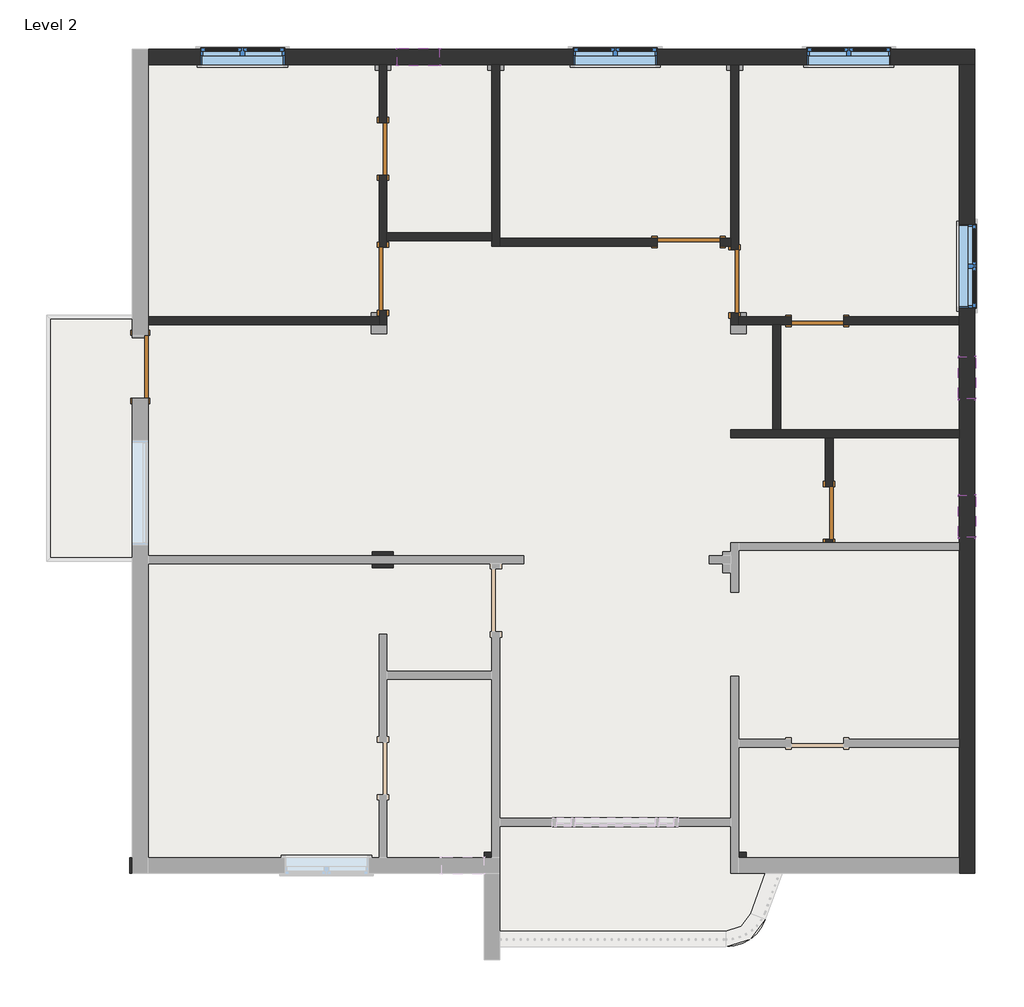
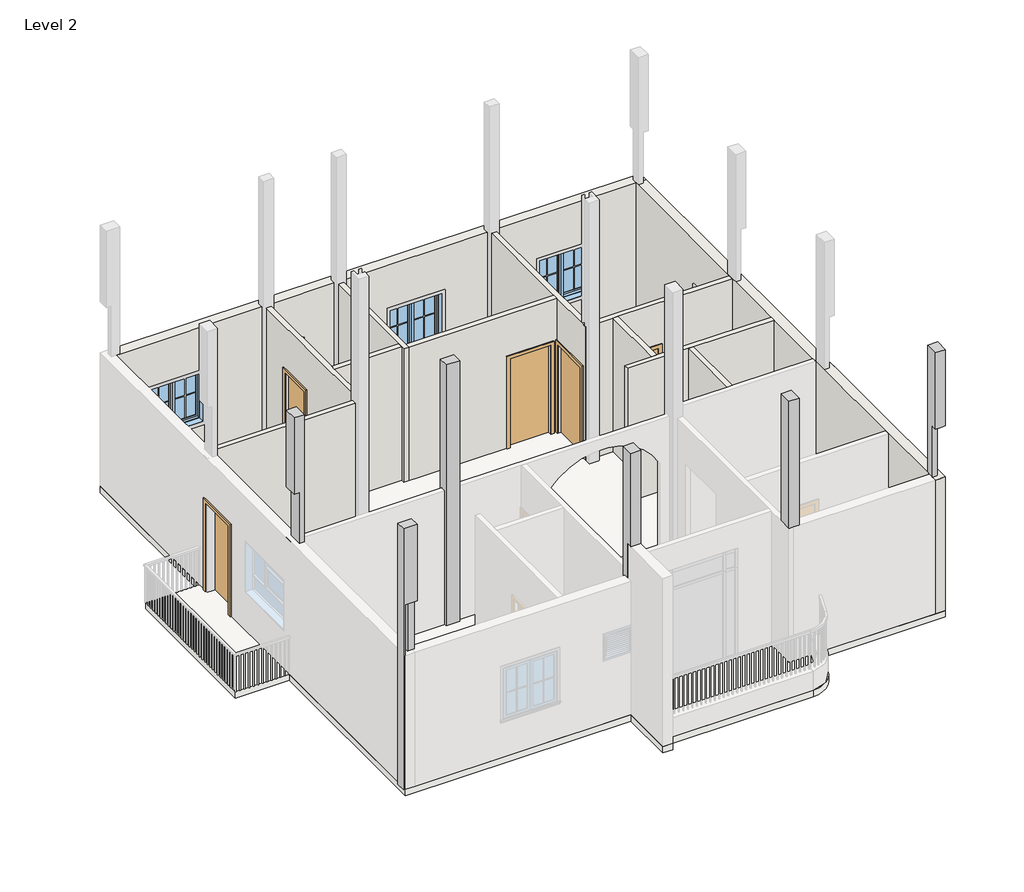
# One storey, part 2 of 4: 12 walls, 7 doors, 7 windows, 6 columns, 1 slab.
"""IFC4 building model written with IfcOpenShell, lengths in millimetres."""

from ifc_helpers import new_model, si_unit, point, frame, frame_2d, origin, place, context, project, spatial, polyline, circle_curve, trimmed, segment, composite_curve, outline, extrude, faceted_brep, transform, mapped, element, save
from components import door_78caadf7, door_214872d5, door_305aa2a5, door_e5f9f3c4, door_a90ba1ad, window_af3140d2, window_f2d8fef0

model = new_model("IFC4")

# Units and contexts
model_context = context("Model", 3, world=origin())
ifc_project = project(units=[si_unit("LENGTHUNIT", "METRE", prefix="MILLI")], contexts=[model_context])

# Site, building, storey
site = spatial("IfcSite", under=ifc_project)
building = spatial("IfcBuilding", under=site)
storey = spatial("IfcBuildingStorey", under=building, Name="Level 2", Elevation=3200.4)

# Columns
placement = place(None, origin())
element("IfcColumn", 1, ObjectType="Rectangular Column : 9\" x 12\"", at=placement, inside=storey, context=model_context, shape_type="Brep", body=[
    faceted_brep([(-14895.9678125, 6235.466018, 3200.4), (-14667.3678125, 6235.466018, 3200.4), (-14667.3678125, 6178.316018, 3200.4), (-14667.3678125, 6064.016018, 3200.4), (-14667.3678125, 5930.666018, 3200.4), (-14895.9678125, 5930.666018, 3200.4), (-14895.9678125, 6235.466018, 6400.8), (-14781.6678125, 6235.466018, 6400.8), (-14781.6678125, 6235.466018, 7620.0), (-14895.9678125, 6235.466018, 7620.0), (-14895.9678125, 6235.466018, 9448.8), (-14667.3678125, 6235.466018, 9448.8), (-14667.3678125, 5930.666018, 9448.8), (-14895.9678125, 5930.666018, 9448.8), (-14895.9678125, 5930.666018, 7620.0), (-14781.6678125, 5930.666018, 7620.0), (-14781.6678125, 5930.666018, 6400.8), (-14895.9678125, 5930.666018, 6400.8)], [[[0, 1, 2, 3, 4, 5]], [[1, 0, 6, 7, 8, 9, 10, 11]], [[4, 3, 2, 1, 11, 12]], [[5, 4, 12, 13, 14, 15, 16, 17]], [[13, 10, 9, 14]], [[11, 10, 13, 12]], [[7, 16, 15, 8]], [[16, 7, 6, 17]], [[8, 15, 14, 9]], [[0, 5, 17, 6]]]),
])
element("IfcColumn", 2, ObjectType="Rectangular Column : 9\" x 12\"", at=placement, inside=storey, context=model_context, shape_type="SweptSolid", body=[
    extrude(outline(polyline([(6006.866018, 3200.4), (6006.866018, 9448.8), (6235.466018, 9448.8), (6235.466018, 3200.4), (6178.316018, 3200.4), (6178.316018, 6400.8), (6064.016018, 6400.8), (6064.016018, 3200.4), (6006.866018, 3200.4)])), frame((-11409.8178125, 0.0, 0.0), z_axis=(1.0, 0.0, 0.0), x_axis=(0.0, 1.0, 0.0)), (0.0, 0.0, 1.0), 304.8),
])
element("IfcColumn", 3, ObjectType="Rectangular Column : 9\" x 12\"", at=placement, inside=storey, context=model_context, shape_type="Brep", body=[
    faceted_brep([(-14934.0678125, 1568.216018, 3200.4), (-14934.0678125, 1796.816018, 3200.4), (-14895.9678125, 1796.816018, 3200.4), (-14895.9678125, 1568.216018, 3200.4), (-14629.2678125, 1796.816018, 9448.8), (-14629.2678125, 1568.216018, 9448.8), (-14629.2678125, 1568.216018, 7620.0), (-14629.2678125, 1682.516018, 7620.0), (-14629.2678125, 1682.516018, 6400.8), (-14629.2678125, 1796.816018, 6400.8), (-14934.0678125, 1568.216018, 9448.8), (-14895.9678125, 1568.216018, 6400.8), (-14895.9678125, 1568.216018, 7620.0), (-14934.0678125, 1796.816018, 9448.8), (-14667.3678125, 1796.816018, 6400.8), (-14781.6678125, 1796.816018, 6400.8), (-14781.6678125, 1796.816018, 7620.0), (-14895.9678125, 1796.816018, 7620.0), (-14895.9678125, 1796.816018, 6400.8), (-14895.9678125, 1682.516018, 6400.8), (-14667.3678125, 1682.516018, 6400.8), (-14781.6678125, 1682.516018, 6400.8), (-14781.6678125, 1682.516018, 7620.0), (-14895.9678125, 1682.516018, 7620.0)], [[[0, 1, 2, 3]], [[4, 5, 6, 7, 8, 9]], [[5, 10, 0, 3, 11, 12, 6]], [[1, 0, 10, 13]], [[1, 13, 4, 9, 14, 15, 16, 17, 18, 2]], [[5, 4, 13, 10]], [[3, 2, 18, 19, 11]], [[14, 20, 21, 15]], [[14, 9, 8, 20]], [[8, 7, 22, 21, 20]], [[7, 6, 12, 23, 22]], [[23, 12, 11, 19]], [[17, 23, 19, 18]], [[22, 16, 15, 21]], [[23, 17, 16, 22]]]),
])
element("IfcColumn", 4, ObjectType="Rectangular Column : 9\" x 12\"", at=placement, inside=storey, context=model_context, shape_type="Brep", body=[
    faceted_brep([(-9561.9678125, 1568.216018, 3200.4), (-9790.5678125, 1568.216018, 3200.4), (-9790.5678125, 1873.016018, 3200.4), (-9676.2678125, 1873.016018, 3200.4), (-9676.2678125, 1796.816018, 3200.4), (-9561.9678125, 1796.816018, 3200.4), (-9790.5678125, 1873.016018, 9448.8), (-9561.9678125, 1873.016018, 9448.8), (-9561.9678125, 1873.016018, 6400.8), (-9676.2678125, 1873.016018, 6400.8), (-9561.9678125, 1568.216018, 9448.8), (-9561.9678125, 1568.216018, 7218.0977729), (-9561.9678125, 1682.516018, 7218.0977729), (-9561.9678125, 1682.516018, 6400.8), (-9561.9678125, 1568.216018, 6400.8), (-9561.9678125, 1796.816018, 6400.8), (-9790.5678125, 1568.216018, 9448.8), (-9790.5678125, 1568.216018, 7620.0), (-9790.5678125, 1568.216018, 7218.0977729), (-9790.5678125, 1568.216018, 6400.8), (-9790.5678125, 1682.516018, 6400.8), (-9790.5678125, 1682.516018, 7218.0977729), (-9676.2678125, 1796.816018, 6400.8)], [[[0, 1, 2, 3, 4, 5]], [[6, 7, 8, 9, 3, 2]], [[7, 10, 11, 12, 13, 14, 0, 5, 15, 8]], [[10, 16, 17, 18, 11]], [[2, 1, 19, 20, 21, 18, 17, 16, 6]], [[7, 6, 16, 10]], [[22, 4, 3, 9]], [[15, 22, 9, 8]], [[4, 22, 15, 5]], [[21, 12, 11, 18]], [[13, 20, 19, 14]], [[12, 21, 20, 13]], [[1, 0, 14, 19]]]),
])
element("IfcColumn", 5, ObjectType="Rectangular Column : 9\" x 12\"", at=placement, inside=storey, context=model_context, shape_type="Brep", body=[
    faceted_brep([(-6094.8678125, 1873.016018, 3200.4), (-5980.5678125, 1873.016018, 3200.4), (-5980.5678125, 1796.816018, 3200.4), (-6094.8678125, 1796.816018, 3200.4), (-6209.1678125, 1873.016018, 9448.8), (-5980.5678125, 1873.016018, 9448.8), (-6094.8678125, 1873.016018, 6400.8), (-6209.1678125, 1873.016018, 6400.8), (-5980.5678125, 1568.216018, 9448.8), (-5980.5678125, 1568.216018, 6400.8), (-5980.5678125, 1796.816018, 6400.8), (-6209.1678125, 1568.216018, 9448.8), (-6209.1678125, 1568.216018, 6400.8), (-6094.8678125, 1568.216018, 6400.8), (-6094.8678125, 1796.816018, 6400.8)], [[[0, 1, 2, 3]], [[4, 5, 1, 0, 6, 7]], [[1, 5, 8, 9, 10, 2]], [[8, 11, 12, 13, 9]], [[11, 4, 7, 12]], [[5, 4, 11, 8]], [[6, 0, 3, 14]], [[7, 6, 14, 13, 12]], [[10, 14, 3, 2]], [[14, 10, 9, 13]]]),
])
element("IfcColumn", 6, ObjectType="Rectangular Column : 9\" x 12\"", at=placement, inside=storey, context=model_context, shape_type="Brep", body=[
    faceted_brep([(-2894.4678125, 1873.016018, 3200.4), (-2665.8678125, 1873.016018, 3200.4), (-2665.8678125, 1568.216018, 3200.4), (-2894.4678125, 1568.216018, 3200.4), (-2894.4678125, 1796.816018, 3200.4), (-2894.4678125, 1873.016018, 9448.8), (-2665.8678125, 1873.016018, 9448.8), (-2665.8678125, 1873.016018, 7620.0), (-2780.1678125, 1873.016018, 7620.0), (-2780.1678125, 1873.016018, 6400.8), (-2665.8678125, 1873.016018, 6400.8), (-2665.8678125, 1568.216018, 9448.8), (-2665.8678125, 1568.216018, 7620.0), (-2894.4678125, 1568.216018, 9448.8), (-2894.4678125, 1568.216018, 7620.0), (-2780.1678125, 1568.216018, 7620.0), (-2894.4678125, 1568.216018, 6400.8), (-2894.4678125, 1682.516018, 6400.8), (-2894.4678125, 1682.516018, 7620.0), (-2780.1678125, 1682.516018, 7620.0), (-2780.1678125, 1682.516018, 6400.8), (-2780.1678125, 1568.216018, 6400.8), (-2665.8678125, 1568.216018, 6400.8)], [[[0, 1, 2, 3, 4]], [[1, 0, 5, 6, 7, 8, 9, 10]], [[6, 11, 12, 7]], [[11, 13, 14, 15, 12]], [[0, 4, 3, 16, 17, 18, 14, 13, 5]], [[6, 5, 13, 11]], [[9, 8, 19, 20]], [[10, 9, 20, 21, 22]], [[8, 7, 12, 15, 19]], [[2, 1, 10, 22]], [[17, 20, 19, 18]], [[20, 17, 16, 21]], [[18, 19, 15, 14]], [[3, 2, 22, 21, 16]]]),
])

# Doors
door_shape = door_78caadf7(model_context)
element("IfcDoor", 7, ObjectType="Single-Flush : 2'6\"x 7'", at=placement, inside=storey, context=model_context, shape_type="MappedRepresentation", body=[
    mapped(door_shape, transform((-11257.4178125, 12083.816018, 3200.4), x_axis=(0.0, 1.0, 0.0), y_axis=(-1.0, 0.0, 0.0), z_axis=(0.0, 0.0, 1.0))),
])
door_2_shape = door_214872d5(model_context)
element("IfcDoor", 8, ObjectType="Single-Flush : 2'6\"x 7'", at=placement, inside=storey, context=model_context, shape_type="MappedRepresentation", body=[
    mapped(door_2_shape, transform((-4951.8678125, 9588.266018, 3200.4), x_axis=(-1.0, 0.0, 0.0), y_axis=(0.0, -1.0, 0.0), z_axis=(0.0, 0.0, 1.0))),
])
element("IfcDoor", 9, ObjectType="Single-Flush : 2'6\"x 7'", at=placement, inside=storey, context=model_context, shape_type="MappedRepresentation", body=[
    mapped(door_2_shape, transform((-4780.4178125, 6800.616018, 3200.4), x_axis=(0.0, -1.0, 0.0), y_axis=(1.0, 0.0, 0.0), z_axis=(0.0, 0.0, 1.0))),
])
door_3_shape = door_305aa2a5(model_context)
element("IfcDoor", 10, ObjectType="Single-Flush : 36\" x 84\"", at=placement, inside=storey, context=model_context, shape_type="MappedRepresentation", body=[
    mapped(door_3_shape, transform((-11257.4178125, 10197.866018, 3200.4), x_axis=(0.0, -1.0, 0.0), y_axis=(1.0, 0.0, 0.0), z_axis=(0.0, 0.0, 1.0))),
])
door_4_shape = door_e5f9f3c4(model_context)
element("IfcDoor", 11, ObjectType="Single-Flush : 36\" x 84\"", at=placement, inside=storey, context=model_context, shape_type="MappedRepresentation", body=[
    mapped(door_4_shape, transform((-6818.7678125, 10731.266018, 3200.4), x_axis=(1.0, 0.0, 0.0), y_axis=(0.0, 1.0, 0.0), z_axis=(0.0, 0.0, 1.0))),
])
element("IfcDoor", 12, ObjectType="Single-Flush : 36\" x 84\"", at=placement, inside=storey, context=model_context, shape_type="MappedRepresentation", body=[
    mapped(door_4_shape, transform((-6152.0178125, 10159.766018, 3200.4), x_axis=(0.0, -1.0, 0.0), y_axis=(1.0, 0.0, 0.0), z_axis=(0.0, 0.0, 1.0))),
])
door_5_shape = door_a90ba1ad(model_context)
element("IfcDoor", 13, ObjectType="Single-Flush : 36\" x 84\"", at=placement, inside=storey, context=model_context, shape_type="MappedRepresentation", body=[
    mapped(door_5_shape, transform((-14781.6678125, 8921.516018, 3200.4), x_axis=(0.0, 1.0, 0.0), y_axis=(-1.0, 0.0, 0.0), z_axis=(0.0, 0.0, 1.0))),
])

# Slab
element("IfcSlab", 14, ObjectType="6\" floor", at=placement, inside=storey, context=model_context, shape_type="SweptSolid", body=[
    extrude(outline(composite_curve([segment(polyline([(-2665.8678125, 13531.616018), (-2665.8678125, 1568.216018), (-5463.3133278, 1568.216018), (-5705.6066674, 902.5205386)]), True, "CONTINUOUS"), segment(trimmed(circle_curve(frame_2d((-6278.443289, 1111.016018)), 609.6), [point((-5705.6066674, 902.5205386))], [point((-6278.443289, 501.416018))], False, "CARTESIAN"), True, "CONTINUOUS"), segment(polyline([(-6278.443289, 501.416018), (-9561.9678125, 501.416018), (-9561.9678125, 310.916018), (-9790.5678125, 310.916018), (-9790.5678125, 1568.216018), (-14895.9678125, 1568.216018), (-14895.9678125, 6121.166018), (-16115.1678125, 6121.166018), (-16115.1678125, 9645.416018), (-14895.9678125, 9645.416018), (-14895.9678125, 13531.616018), (-2665.8678125, 13531.616018)]), True, "CONTINUOUS")], self_intersect=False)), frame((0.0, 0.0, 3048.0), z_axis=(0.0, 0.0, 1.0), x_axis=(1.0, 0.0, 0.0)), (0.0, 0.0, 1.0), 152.4),
])

# Walls
element("IfcWall", 15, ObjectType="4.5\" wall", at=placement, inside=storey, context=model_context, shape_type="Brep", body=[
    faceted_brep([(-11314.5678125, 9740.666018, 5334.0), (-11314.5678125, 9740.666018, 3200.4), (-11314.5678125, 9702.566018, 3200.4), (-11314.5678125, 9645.416018, 3200.4), (-11314.5678125, 9531.116018, 3200.4), (-11314.5678125, 9531.116018, 6400.8), (-11314.5678125, 9645.416018, 6400.8), (-11314.5678125, 9702.566018, 6400.8), (-11314.5678125, 13226.816018, 6400.8), (-11314.5678125, 13303.016018, 6400.8), (-11314.5678125, 13303.016018, 3200.4), (-11314.5678125, 13226.816018, 3200.4), (-11314.5678125, 12464.816018, 3200.4), (-11314.5678125, 12464.816018, 5334.0), (-11314.5678125, 11702.816018, 5334.0), (-11314.5678125, 11702.816018, 3200.4), (-11314.5678125, 10655.066018, 3200.4), (-11314.5678125, 10655.066018, 5334.0), (-11200.2678125, 9531.116018, 3200.4), (-11200.2678125, 9740.666018, 3200.4), (-11200.2678125, 9740.666018, 5334.0), (-11200.2678125, 10655.066018, 5334.0), (-11200.2678125, 10655.066018, 3200.4), (-11200.2678125, 10750.316018, 3200.4), (-11200.2678125, 10864.616018, 3200.4), (-11200.2678125, 11702.816018, 3200.4), (-11200.2678125, 11702.816018, 5334.0), (-11200.2678125, 12464.816018, 5334.0), (-11200.2678125, 12464.816018, 3200.4), (-11200.2678125, 13226.816018, 3200.4), (-11200.2678125, 13303.016018, 3200.4), (-11200.2678125, 13303.016018, 6400.8), (-11200.2678125, 13226.816018, 6400.8), (-11200.2678125, 10864.616018, 6400.8), (-11200.2678125, 10750.316018, 6400.8), (-11200.2678125, 9702.566018, 6400.8), (-11200.2678125, 9683.516018, 6400.8), (-11200.2678125, 9569.216018, 6400.8), (-11200.2678125, 9531.116018, 6400.8)], [[[0, 1, 2, 3, 4, 5, 6, 7, 8, 9, 10, 11, 12, 13, 14, 15, 16, 17]], [[18, 19, 20, 21, 22, 23, 24, 25, 26, 27, 28, 29, 30, 31, 32, 33, 34, 35, 36, 37, 38]], [[16, 15, 25, 24, 23, 22]], [[4, 3, 2, 1, 19, 18]], [[30, 29, 28, 12, 11, 10]], [[9, 8, 7, 6, 5, 38, 37, 36, 35, 34, 33, 32, 31]], [[10, 9, 31, 30]], [[5, 4, 18, 38]], [[13, 12, 28, 27]], [[14, 13, 27, 26]], [[15, 14, 26, 25]], [[20, 19, 1, 0]], [[21, 20, 0, 17]], [[22, 21, 17, 16]]]),
])
element("IfcWall", 16, ObjectType="4.5\" wall", at=placement, inside=storey, context=model_context, shape_type="Brep", body=[
    faceted_brep([(-14667.3678125, 9531.116018, 3200.4), (-11428.8678125, 9531.116018, 3200.4), (-11314.5678125, 9531.116018, 3200.4), (-11314.5678125, 9531.116018, 6400.8), (-11428.8678125, 9531.116018, 6400.8), (-14667.3678125, 9531.116018, 6400.8), (-14667.3678125, 9645.416018, 3200.4), (-14667.3678125, 9645.416018, 6400.8), (-11428.8678125, 9645.416018, 6400.8), (-11371.7178125, 9645.416018, 6400.8), (-11314.5678125, 9645.416018, 6400.8), (-11314.5678125, 9645.416018, 3200.4), (-11428.8678125, 9645.416018, 3200.4)], [[[0, 1, 2, 3, 4, 5]], [[6, 7, 8, 9, 10, 11, 12]], [[2, 1, 0, 6, 12, 11]], [[5, 4, 3, 10, 9, 8, 7]], [[0, 5, 7, 6]], [[3, 2, 11, 10]]]),
])
element("IfcWall", 17, ObjectType="4.5\" wall", at=placement, inside=storey, context=model_context, shape_type="Brep", body=[
    faceted_brep([(-9676.2678125, 13303.016018, 3200.4), (-9676.2678125, 13226.816018, 3200.4), (-9676.2678125, 10864.616018, 3200.4), (-9676.2678125, 10750.316018, 3200.4), (-9676.2678125, 10674.116018, 3200.4), (-9676.2678125, 10674.116018, 6400.8), (-9676.2678125, 10750.316018, 6400.8), (-9676.2678125, 10864.616018, 6400.8), (-9676.2678125, 13226.816018, 6400.8), (-9676.2678125, 13303.016018, 6400.8), (-9561.9678125, 13303.016018, 3200.4), (-9561.9678125, 13303.016018, 6400.8), (-9561.9678125, 13226.816018, 6400.8), (-9561.9678125, 10788.416018, 6400.8), (-9561.9678125, 10674.116018, 6400.8), (-9561.9678125, 10674.116018, 3200.4), (-9561.9678125, 10788.416018, 3200.4), (-9561.9678125, 13226.816018, 3200.4)], [[[0, 1, 2, 3, 4, 5, 6, 7, 8, 9]], [[10, 11, 12, 13, 14, 15, 16, 17]], [[4, 3, 2, 1, 0, 10, 17, 16, 15]], [[9, 8, 7, 6, 5, 14, 13, 12, 11]], [[0, 9, 11, 10]], [[5, 4, 15, 14]]]),
])
element("IfcWall", 18, ObjectType="4.5\" wall", at=placement, inside=storey, context=model_context, shape_type="SweptSolid", body=[
    extrude(outline(polyline([(-9676.2678125, 10750.316018), (-11200.2678125, 10750.316018), (-11200.2678125, 10864.616018), (-9676.2678125, 10864.616018), (-9676.2678125, 10750.316018)])), frame((0.0, 0.0, 3200.4), z_axis=(0.0, 0.0, 1.0), x_axis=(1.0, 0.0, 0.0)), (0.0, 0.0, 1.0), 3200.4),
])
element("IfcWall", 19, ObjectType="4.5\" wall", at=placement, inside=storey, context=model_context, shape_type="Brep", body=[
    faceted_brep([(-6209.1678125, 9702.566018, 5334.0), (-6209.1678125, 9702.566018, 3200.4), (-6209.1678125, 9531.116018, 3200.4), (-6209.1678125, 9531.116018, 6400.8), (-6209.1678125, 9569.216018, 6400.8), (-6209.1678125, 9683.516018, 6400.8), (-6209.1678125, 9702.566018, 6400.8), (-6209.1678125, 10674.116018, 6400.8), (-6209.1678125, 10788.416018, 6400.8), (-6209.1678125, 13226.816018, 6400.8), (-6209.1678125, 13303.016018, 6400.8), (-6209.1678125, 13303.016018, 3200.4), (-6209.1678125, 13226.816018, 3200.4), (-6209.1678125, 10788.416018, 3200.4), (-6209.1678125, 10674.116018, 3200.4), (-6209.1678125, 10616.966018, 3200.4), (-6209.1678125, 10616.966018, 5334.0), (-6094.8678125, 9531.116018, 3200.4), (-6094.8678125, 9645.416018, 3200.4), (-6094.8678125, 9702.566018, 3200.4), (-6094.8678125, 9702.566018, 5334.0), (-6094.8678125, 10616.966018, 5334.0), (-6094.8678125, 10616.966018, 3200.4), (-6094.8678125, 13226.816018, 3200.4), (-6094.8678125, 13303.016018, 3200.4), (-6094.8678125, 13303.016018, 6400.8), (-6094.8678125, 13226.816018, 6400.8), (-6094.8678125, 9702.566018, 6400.8), (-6094.8678125, 9683.516018, 6400.8), (-6094.8678125, 9645.416018, 6400.8), (-6094.8678125, 9531.116018, 6400.8)], [[[0, 1, 2, 3, 4, 5, 6, 7, 8, 9, 10, 11, 12, 13, 14, 15, 16]], [[17, 18, 19, 20, 21, 22, 23, 24, 25, 26, 27, 28, 29, 30]], [[2, 1, 19, 18, 17]], [[15, 14, 13, 12, 11, 24, 23, 22]], [[10, 9, 8, 7, 6, 5, 4, 3, 30, 29, 28, 27, 26, 25]], [[11, 10, 25, 24]], [[3, 2, 17, 30]], [[20, 19, 1, 0]], [[21, 20, 0, 16]], [[22, 21, 16, 15]]]),
])
element("IfcWall", 20, ObjectType="4.5\" wall", at=placement, inside=storey, context=model_context, shape_type="SweptSolid", body=[
    extrude(outline(polyline([(5334.0, -6361.5678125), (3200.4, -6361.5678125), (3200.4, -6209.1678125), (6400.8, -6209.1678125), (6400.8, -9561.9678125), (3200.4, -9561.9678125), (3200.4, -7275.9678125), (5334.0, -7275.9678125), (5334.0, -6361.5678125)])), frame((0.0, 10674.116018, 0.0), z_axis=(0.0, 1.0, 0.0), x_axis=(0.0, 0.0, 1.0)), (0.0, 0.0, 1.0), 114.3),
])
element("IfcWall", 21, ObjectType="4.5\" wall", at=placement, inside=storey, context=model_context, shape_type="Brep", body=[
    faceted_brep([(-6094.8678125, 9531.116018, 3200.4), (-5980.5678125, 9531.116018, 3200.4), (-5599.5678125, 9531.116018, 3200.4), (-5485.2678125, 9531.116018, 3200.4), (-5332.8678125, 9531.116018, 3200.4), (-5332.8678125, 9531.116018, 5334.0), (-4570.8678125, 9531.116018, 5334.0), (-4570.8678125, 9531.116018, 3200.4), (-2894.4678125, 9531.116018, 3200.4), (-2894.4678125, 9531.116018, 6400.8), (-5485.2678125, 9531.116018, 6400.8), (-5599.5678125, 9531.116018, 6400.8), (-5980.5678125, 9531.116018, 6400.8), (-6094.8678125, 9531.116018, 6400.8), (-5332.8678125, 9645.416018, 5334.0), (-5332.8678125, 9645.416018, 3200.4), (-5980.5678125, 9645.416018, 3200.4), (-6094.8678125, 9645.416018, 3200.4), (-6094.8678125, 9645.416018, 6400.8), (-6037.7178125, 9645.416018, 6400.8), (-5980.5678125, 9645.416018, 6400.8), (-2894.4678125, 9645.416018, 6400.8), (-2894.4678125, 9645.416018, 3200.4), (-4570.8678125, 9645.416018, 3200.4), (-4570.8678125, 9645.416018, 5334.0)], [[[0, 1, 2, 3, 4, 5, 6, 7, 8, 9, 10, 11, 12, 13]], [[14, 15, 16, 17, 18, 19, 20, 21, 22, 23, 24]], [[23, 22, 8, 7]], [[17, 16, 15, 4, 3, 2, 1, 0]], [[13, 12, 11, 10, 9, 21, 20, 19, 18]], [[0, 13, 18, 17]], [[9, 8, 22, 21]], [[5, 4, 15, 14]], [[6, 5, 14, 24]], [[7, 6, 24, 23]]]),
])
element("IfcWall", 22, ObjectType="4.5\" wall", at=placement, inside=storey, context=model_context, shape_type="Brep", body=[
    faceted_brep([(-2894.4678125, 8007.116018, 3200.4), (-5485.2678125, 8007.116018, 3200.4), (-5599.5678125, 8007.116018, 3200.4), (-6209.1678125, 8007.116018, 3200.4), (-6209.1678125, 8007.116018, 6400.8), (-5599.5678125, 8007.116018, 6400.8), (-5485.2678125, 8007.116018, 6400.8), (-2894.4678125, 8007.116018, 6400.8), (-2894.4678125, 7892.816018, 3200.4), (-2894.4678125, 7892.816018, 6400.8), (-4723.2678125, 7892.816018, 6400.8), (-4837.5678125, 7892.816018, 6400.8), (-6209.1678125, 7892.816018, 6400.8), (-6209.1678125, 7892.816018, 3200.4), (-4837.5678125, 7892.816018, 3200.4), (-4723.2678125, 7892.816018, 3200.4)], [[[0, 1, 2, 3, 4, 5, 6, 7]], [[8, 9, 10, 11, 12, 13, 14, 15]], [[3, 2, 1, 0, 8, 15, 14, 13]], [[4, 3, 13, 12]], [[7, 6, 5, 4, 12, 11, 10, 9]], [[0, 7, 9, 8]]]),
])
element("IfcWall", 23, ObjectType="4.5\" wall", at=placement, inside=storey, context=model_context, shape_type="SweptSolid", body=[
    extrude(outline(polyline([(-5599.5678125, 8007.116018), (-5599.5678125, 9531.116018), (-5485.2678125, 9531.116018), (-5485.2678125, 8007.116018), (-5599.5678125, 8007.116018)])), frame((0.0, 0.0, 3200.4), z_axis=(0.0, 0.0, 1.0), x_axis=(1.0, 0.0, 0.0)), (0.0, 0.0, 1.0), 3200.4),
])
element("IfcWall", 24, ObjectType="4.5\" wall", at=placement, inside=storey, context=model_context, shape_type="SweptSolid", body=[
    extrude(outline(polyline([(6419.616018, 5334.0), (6419.616018, 3200.4), (6368.816018, 3200.4), (6368.816018, 6400.8), (7892.816018, 6400.8), (7892.816018, 3200.4), (7181.616018, 3200.4), (7181.616018, 5334.0), (6419.616018, 5334.0)])), frame((-4837.5678125, 0.0, 0.0), z_axis=(1.0, 0.0, 0.0), x_axis=(0.0, 1.0, 0.0)), (0.0, 0.0, 1.0), 114.3),
])
element("IfcWall", 25, ObjectType="9\" wall", at=placement, inside=storey, context=model_context, shape_type="Brep", body=[
    faceted_brep([(-14667.3678125, 13303.016018, 3200.4), (-14591.1678125, 13303.016018, 3200.4), (-11371.7178125, 13303.016018, 3200.4), (-11314.5678125, 13303.016018, 3200.4), (-11200.2678125, 13303.016018, 3200.4), (-11143.1178125, 13303.016018, 3200.4), (-9733.4178125, 13303.016018, 3200.4), (-9676.2678125, 13303.016018, 3200.4), (-9561.9678125, 13303.016018, 3200.4), (-9504.8178125, 13303.016018, 3200.4), (-6266.3178125, 13303.016018, 3200.4), (-6209.1678125, 13303.016018, 3200.4), (-6094.8678125, 13303.016018, 3200.4), (-6037.7178125, 13303.016018, 3200.4), (-2894.4678125, 13303.016018, 3200.4), (-2665.8678125, 13303.016018, 3200.4), (-2665.8678125, 13303.016018, 6400.8), (-2780.1678125, 13303.016018, 6400.8), (-2894.4678125, 13303.016018, 6400.8), (-6037.7178125, 13303.016018, 6400.8), (-6094.8678125, 13303.016018, 6400.8), (-6209.1678125, 13303.016018, 6400.8), (-6266.3178125, 13303.016018, 6400.8), (-9504.8178125, 13303.016018, 6400.8), (-9561.9678125, 13303.016018, 6400.8), (-9676.2678125, 13303.016018, 6400.8), (-9733.4178125, 13303.016018, 6400.8), (-11143.1178125, 13303.016018, 6400.8), (-11200.2678125, 13303.016018, 6400.8), (-11314.5678125, 13303.016018, 6400.8), (-11371.7178125, 13303.016018, 6400.8), (-14591.1678125, 13303.016018, 6400.8), (-14667.3678125, 13303.016018, 6400.8), (-10438.2678125, 13303.016018, 5334.0), (-10438.2678125, 13303.016018, 4724.4), (-11047.8678125, 13303.016018, 4724.4), (-11047.8678125, 13303.016018, 5334.0), (-12686.1678125, 13303.016018, 5334.0), (-12686.1678125, 13303.016018, 4114.8), (-13905.3678125, 13303.016018, 4114.8), (-13905.3678125, 13303.016018, 5334.0), (-7275.9678125, 13303.016018, 5334.0), (-7275.9678125, 13303.016018, 4114.8), (-8495.1678125, 13303.016018, 4114.8), (-8495.1678125, 13303.016018, 5334.0), (-3885.0678125, 13303.016018, 5334.0), (-3885.0678125, 13303.016018, 4114.8), (-5104.2678125, 13303.016018, 4114.8), (-5104.2678125, 13303.016018, 5334.0), (-14667.3678125, 13531.616018, 3200.4), (-14667.3678125, 13531.616018, 6400.8), (-2665.8678125, 13531.616018, 6400.8), (-2665.8678125, 13531.616018, 3200.4), (-14591.1678125, 13531.616018, 3200.4), (-10438.2678125, 13531.616018, 5334.0), (-11047.8678125, 13531.616018, 5334.0), (-11047.8678125, 13531.616018, 4724.4), (-10438.2678125, 13531.616018, 4724.4), (-12686.1678125, 13531.616018, 5334.0), (-13905.3678125, 13531.616018, 5334.0), (-13905.3678125, 13531.616018, 4114.8), (-12686.1678125, 13531.616018, 4114.8), (-7275.9678125, 13531.616018, 5334.0), (-8495.1678125, 13531.616018, 5334.0), (-8495.1678125, 13531.616018, 4114.8), (-7275.9678125, 13531.616018, 4114.8), (-3885.0678125, 13531.616018, 5334.0), (-5104.2678125, 13531.616018, 5334.0), (-5104.2678125, 13531.616018, 4114.8), (-3885.0678125, 13531.616018, 4114.8)], [[[0, 1, 2, 3, 4, 5, 6, 7, 8, 9, 10, 11, 12, 13, 14, 15, 16, 17, 18, 19, 20, 21, 22, 23, 24, 25, 26, 27, 28, 29, 30, 31, 32], [33, 34, 35, 36], [37, 38, 39, 40], [41, 42, 43, 44], [45, 46, 47, 48]], [[49, 50, 51, 52, 53], [54, 55, 56, 57], [58, 59, 60, 61], [62, 63, 64, 65], [66, 67, 68, 69]], [[15, 14, 13, 12, 11, 10, 9, 8, 7, 6, 5, 4, 3, 2, 1, 0, 49, 53, 52]], [[32, 31, 30, 29, 28, 27, 26, 25, 24, 23, 22, 21, 20, 19, 18, 17, 16, 51, 50]], [[0, 32, 50, 49]], [[16, 15, 52, 51]], [[34, 33, 54, 57]], [[35, 34, 57, 56]], [[36, 35, 56, 55]], [[33, 36, 55, 54]], [[38, 37, 58, 61]], [[39, 38, 61, 60]], [[40, 39, 60, 59]], [[37, 40, 59, 58]], [[42, 41, 62, 65]], [[43, 42, 65, 64]], [[44, 43, 64, 63]], [[41, 44, 63, 62]], [[46, 45, 66, 69]], [[47, 46, 69, 68]], [[48, 47, 68, 67]], [[45, 48, 67, 66]]]),
])
element("IfcWall", 26, ObjectType="9\" wall", at=placement, inside=storey, context=model_context, shape_type="Brep", body=[
    faceted_brep([(-2894.4678125, 13303.016018, 3200.4), (-2894.4678125, 13226.816018, 3200.4), (-2894.4678125, 9702.566018, 3200.4), (-2894.4678125, 9645.416018, 3200.4), (-2894.4678125, 9531.116018, 3200.4), (-2894.4678125, 9397.766018, 3200.4), (-2894.4678125, 8007.116018, 3200.4), (-2894.4678125, 7892.816018, 3200.4), (-2894.4678125, 6368.816018, 3200.4), (-2894.4678125, 6254.516018, 3200.4), (-2894.4678125, 6235.466018, 3200.4), (-2894.4678125, 5930.666018, 3200.4), (-2894.4678125, 3511.316018, 3200.4), (-2894.4678125, 3397.016018, 3200.4), (-2894.4678125, 1873.016018, 3200.4), (-2894.4678125, 1796.816018, 3200.4), (-2894.4678125, 1568.216018, 3200.4), (-2894.4678125, 1568.216018, 6400.8), (-2894.4678125, 1682.516018, 6400.8), (-2894.4678125, 1796.816018, 6400.8), (-2894.4678125, 1873.016018, 6400.8), (-2894.4678125, 3397.016018, 6400.8), (-2894.4678125, 3511.316018, 6400.8), (-2894.4678125, 5930.666018, 6400.8), (-2894.4678125, 6235.466018, 6400.8), (-2894.4678125, 6254.516018, 6400.8), (-2894.4678125, 6368.816018, 6400.8), (-2894.4678125, 7892.816018, 6400.8), (-2894.4678125, 8007.116018, 6400.8), (-2894.4678125, 9397.766018, 6400.8), (-2894.4678125, 9531.116018, 6400.8), (-2894.4678125, 9645.416018, 6400.8), (-2894.4678125, 9702.566018, 6400.8), (-2894.4678125, 13226.816018, 6400.8), (-2894.4678125, 13303.016018, 6400.8), (-2894.4678125, 7054.616018, 5334.0), (-2894.4678125, 6445.016018, 5334.0), (-2894.4678125, 6445.016018, 4724.4), (-2894.4678125, 7054.616018, 4724.4), (-2894.4678125, 9064.391018, 5334.0), (-2894.4678125, 8454.791018, 5334.0), (-2894.4678125, 8454.791018, 4724.4), (-2894.4678125, 9064.391018, 4724.4), (-2894.4678125, 9772.416018, 5334.0), (-2894.4678125, 9772.416018, 4114.8), (-2894.4678125, 10991.616018, 4114.8), (-2894.4678125, 10991.616018, 5334.0), (-2665.8678125, 13303.016018, 3200.4), (-2665.8678125, 13303.016018, 6400.8), (-2665.8678125, 1568.216018, 6400.8), (-2665.8678125, 1568.216018, 3200.4), (-2665.8678125, 1873.016018, 3200.4), (-2665.8678125, 5930.666018, 3200.4), (-2665.8678125, 6235.466018, 3200.4), (-2665.8678125, 9397.766018, 3200.4), (-2665.8678125, 9702.566018, 3200.4), (-2665.8678125, 13226.816018, 3200.4), (-2665.8678125, 7054.616018, 5334.0), (-2665.8678125, 7054.616018, 4724.4), (-2665.8678125, 6445.016018, 4724.4), (-2665.8678125, 6445.016018, 5334.0), (-2665.8678125, 9064.391018, 5334.0), (-2665.8678125, 9064.391018, 4724.4), (-2665.8678125, 8454.791018, 4724.4), (-2665.8678125, 8454.791018, 5334.0), (-2665.8678125, 9772.416018, 5334.0), (-2665.8678125, 10991.616018, 5334.0), (-2665.8678125, 10991.616018, 4114.8), (-2665.8678125, 9772.416018, 4114.8)], [[[0, 1, 2, 3, 4, 5, 6, 7, 8, 9, 10, 11, 12, 13, 14, 15, 16, 17, 18, 19, 20, 21, 22, 23, 24, 25, 26, 27, 28, 29, 30, 31, 32, 33, 34], [35, 36, 37, 38], [39, 40, 41, 42], [43, 44, 45, 46]], [[47, 48, 49, 50, 51, 52, 53, 54, 55, 56], [57, 58, 59, 60], [61, 62, 63, 64], [65, 66, 67, 68]], [[16, 15, 14, 13, 12, 11, 10, 9, 8, 7, 6, 5, 4, 3, 2, 1, 0, 47, 56, 55, 54, 53, 52, 51, 50]], [[34, 33, 32, 31, 30, 29, 28, 27, 26, 25, 24, 23, 22, 21, 20, 19, 18, 17, 49, 48]], [[0, 34, 48, 47]], [[17, 16, 50, 49]], [[58, 57, 35, 38]], [[59, 58, 38, 37]], [[60, 59, 37, 36]], [[57, 60, 36, 35]], [[62, 61, 39, 42]], [[63, 62, 42, 41]], [[64, 63, 41, 40]], [[61, 64, 40, 39]], [[44, 43, 65, 68]], [[45, 44, 68, 67]], [[46, 45, 67, 66]], [[43, 46, 66, 65]]]),
])

# Windows
window_shape = window_af3140d2(model_context)
element("IfcWindow", 27, ObjectType="Window-Casement-Double : 48\" x 48\"", at=placement, inside=storey, context=model_context, shape_type="MappedRepresentation", body=[
    mapped(window_shape, transform((-13295.7678125, 13417.316018, 3200.4), x_axis=(1.0, 0.0, 0.0), y_axis=(0.0, 1.0, 0.0), z_axis=(0.0, 0.0, 1.0))),
])
element("IfcWindow", 28, ObjectType="Window-Casement-Double : 48\" x 48\"", at=placement, inside=storey, context=model_context, shape_type="MappedRepresentation", body=[
    mapped(window_shape, transform((-7885.5678125, 13417.316018, 3200.4), x_axis=(1.0, 0.0, 0.0), y_axis=(0.0, 1.0, 0.0), z_axis=(0.0, 0.0, 1.0))),
])
element("IfcWindow", 29, ObjectType="Window-Casement-Double : 48\" x 48\"", at=placement, inside=storey, context=model_context, shape_type="MappedRepresentation", body=[
    mapped(window_shape, transform((-4494.6678125, 13417.316018, 3200.4), x_axis=(1.0, 0.0, 0.0), y_axis=(0.0, 1.0, 0.0), z_axis=(0.0, 0.0, 1.0))),
])
element("IfcWindow", 30, ObjectType="Window-Casement-Double : 48\" x 48\"", at=placement, inside=storey, context=model_context, shape_type="MappedRepresentation", body=[
    mapped(window_shape, transform((-2780.1678125, 10382.016018, 3200.4), x_axis=(0.0, -1.0, 0.0), y_axis=(1.0, 0.0, 0.0), z_axis=(0.0, 0.0, 1.0))),
])
window_2_shape = window_f2d8fef0(model_context)
element("IfcWindow", 31, ObjectType="Window-Louvers : 24\" x 24\"", at=placement, inside=storey, context=model_context, shape_type="MappedRepresentation", body=[
    mapped(window_2_shape, transform((-2773.8178125, 6749.816018, 3810.0), x_axis=(0.0, -1.0, 0.0), y_axis=(1.0, 0.0, 0.0), z_axis=(0.0, 0.0, 1.0))),
])
element("IfcWindow", 32, ObjectType="Window-Louvers : 24\" x 24\"", at=placement, inside=storey, context=model_context, shape_type="MappedRepresentation", body=[
    mapped(window_2_shape, transform((-2773.8178125, 8759.591018, 3810.0), x_axis=(0.0, -1.0, 0.0), y_axis=(1.0, 0.0, 0.0), z_axis=(0.0, 0.0, 1.0))),
])
element("IfcWindow", 33, ObjectType="Window-Louvers : 24\" x 24\"", at=placement, inside=storey, context=model_context, shape_type="MappedRepresentation", body=[
    mapped(window_2_shape, transform((-10743.0678125, 13410.966018, 3810.0), x_axis=(-1.0, 0.0, 0.0), y_axis=(0.0, -1.0, 0.0), z_axis=(0.0, 0.0, 1.0))),
])

save(model, "model.ifc")

# Revit data of these elements
# Type "Rectangular Column : 9\" x 12\""
#   Assembly Code = "B1010200"
#   Depth = 0' - 9"
#   Offset Base = 0' - 0"
#   Offset Top = 0' - 0"
#   Width = 1' - 0"
#   Material = none
# Type "Single-Flush : 2'6\"x 7'"
#   Type Mark = "8"
#   Construction Type Id = "MDOOR"
#   Assembly Code = "C1020"
#   Analytic Construction = "Metal"
#   Thickness = 0' - 2"
#   Heat Transfer Coefficient (U) = 0.651978 BTU/(h·ft²·°F)
#   Height = 7' - 0"
#   Trim Projection Ext = 0' - 1"
#   Trim Projection Int = 0' - 1"
#   Trim Width = 0' - 3"
#   Width = 2' - 6"
#   Define Thermal Properties by = 1
#   Door Material = Door - Panel
#   Frame Material = Door - Frame
#   Visual Light Transmittance = 0
#   Solar Heat Gain Coefficient = 0
#   Function = (empty or 0)
#   Wall Closure = (empty or 0)
# Type "Single-Flush : 36\" x 84\""
#   Type Mark = "1"
#   Construction Type Id = "MDOOR"
#   Assembly Code = "C1020"
#   Analytic Construction = "Metal"
#   Thickness = 0' - 2"
#   Heat Transfer Coefficient (U) = 0.651978 BTU/(h·ft²·°F)
#   Height = 7' - 0"
#   Trim Projection Ext = 0' - 1"
#   Trim Projection Int = 0' - 1"
#   Trim Width = 0' - 3"
#   Width = 3' - 0"
#   Define Thermal Properties by = 1
#   Define Thermal Properties by = 1
#   Door Material = Door - Panel
#   Frame Material = Door - Frame
#   Visual Light Transmittance = 0
#   Solar Heat Gain Coefficient = 0
#   Function = (empty or 0)
#   Wall Closure = (empty or 0)
# Type "6\" floor"
#   Assembly Code = "B1010"
#   Function = 0
#   Layers, outside or top first: 0' - 6" "Gypsum Wall Board" (function 1)
# Type "4.5\" wall"
#   Assembly Code = "B2010"
#   Layers, outside or top first: 0' - 4 1/2" "Gypsum Wall Board" (function 1)
# Type "9\" wall"
#   Assembly Code = "B2010"
#   Layers, outside or top first: 0' - 9" "Gypsum Wall Board" (function 1)
# Type "Window-Casement-Double : 48\" x 48\""
#   Type Mark = "16"
#   Fire Rating = "0.5h"
#   Assembly Code = "B2020100"
#   Analytic Construction = "Double glazing - domestic"
#   Frame Extension [instance default] = 0' - 0 1/4"
#   Window Inset [instance default] = 0' - 0"
#   Wall Thickness [instance default] = 0' - 6"
#   Interior Wall Closure [instance default] = 0' - 2 1/4"
#   Half Width = 2' - 0"
#   Visual Light Transmittance = 0.81
#   Thermal Resistance (R) = 1.8146 (h·ft²·°F)/BTU
#   Solar Heat Gain Coefficient = 0.76
#   Rough Width = 4' - 0 1/2"
#   Rough Height = 4' - 0 1/2"
#   Height = 4' - 0"
#   Heat Transfer Coefficient (U) = 0.5511 BTU/(h·ft²·°F)
#   Exterior Wall Closure [instance default] = 0' - 1 1/4"
#   Extension Jamb [instance default] = 0' - 2 1/4"
#   Default Sill Height = 3' - 0"
#   Width = 4' - 0"
#   Define Thermal Properties by = 0
#   Muntin Visibility = yes
#   Interior Trim Visibility [instance default] = yes
#   Exterior Trim Visibility [instance default] = yes
#   Extension Jamb Visibility [instance default] = yes
#   Interior Trim Material = Wood - Stained
#   Muntin Pattern = Muntin Pattern_2x2 : Muntin Pattern_2x2
#   Interior Trim = Trim-Window-Interior-Flat : Picture Frame
#   Interior Frame Material = Wood - Stained
#   Glass Panel Material = Glass
#   Exterior Trim Material = Clad - White
#   Exterior Trim = Trim-Window-Exterior-Flat : with Sill
#   Exterior Frame Material = Clad - White
#   Wall Closure = (empty or 0)
# Type "Window-Louvers : 24\" x 24\""
#   Type Mark = "18"
#   Construction Type Id = "GSP4R"
#   Assembly Code = "B20"
#   Analytic Construction = "1/8 in Pilkington single glazing"
#   Visual Light Transmittance = 0.9
#   Thermal Resistance (R) = 1.53941 (h·ft²·°F)/BTU
#   Solar Heat Gain Coefficient = 0.78
#   Max Height = 1' - 11.74264"
#   Height = 2' - 0"
#   Heat Transfer Coefficient (U) = 0.6496 BTU/(h·ft²·°F)
#   Blade Width [instance default] = 1' - 10 1/2"
#   Blade Vertical Thickness = 0' - 0.35355"
#   Blade Thickness = 0' - 0 1/4"
#   Blade Spacing = 0' - 1 1/2"
#   Blade Height = 0' - 1.85355"
#   Blade Depth = 0' - 3"
#   Blade Angle = 45.00°
#   Default Sill Height = 3' - 0"
#   Trim Projection_Exterior = 0' - 0 1/2"
#   Trim Projection_Interior = 0' - 0 1/2"
#   Trim Width_Exterior = 0' - 1 1/2"
#   Trim Width_Interior = 0' - 1 1/2"
#   Width = 2' - 0"
#   Max Blade Count = 12
#   Define Thermal Properties by = 1
#   Blade Count = 12
#   Frame Material = Birch
#   Louver Material = Birch
#   Trim Exterior Material = Birch
#   Trim Interior Material = Birch
#   Wall Closure = (empty or 0)
# Elements 1, 2, 3, 4, 5, 6 (IfcColumn, "Rectangular Column : 9\" x 12\"")
#   Phase Created = New Construction
#   Materials on its faces: "Gypsum Wall Board"
# Elements 7, 8, 9 (IfcDoor, "Single-Flush : 2'6\"x 7'")
#   Phase Created = New Construction
#   Materials on its faces: "Door - Frame", "Door - Panel"
# Elements 10, 11, 12, 13 (IfcDoor, "Single-Flush : 36\" x 84\"")
#   Phase Created = New Construction
#   Materials on its faces: "Door - Frame", "Door - Panel"
# Element 14 (IfcSlab, "6\" floor")
#   Height Offset From Level = 0' - 0"
#   Phase Created = New Construction
#   Materials on its faces: "Gypsum Wall Board"
# Elements 15, 16, 17, 18, 19, 20, 21, 22, 23, 24 (IfcWall, "4.5\" wall")
#   Top Offset = 0' - 0"
#   Base Offset = 0' - 0"
#   wall height = 10' - 6"
#   Phase Created = New Construction
#   Base Constraint = Level 2
#   Top Constraint = Level 3
#   Materials on its faces: "Gypsum Wall Board"
# Elements 25, 26 (IfcWall, "9\" wall")
#   Top Offset = 0' - 0"
#   Base Offset = 0' - 0"
#   wall height = 10' - 6"
#   Phase Created = New Construction
#   Base Constraint = Level 2
#   Top Constraint = Level 3
#   Materials on its faces: "Gypsum Wall Board"
# Element 27 (IfcWindow, "Window-Casement-Double : 48\" x 48\"")
#   Mark = "16"
#   Window Inset = 0' - 0"
#   Interior Wall Closure = 0' - 2 1/4"
#   Frame Extension = 0' - 0 1/4"
#   Exterior Wall Closure = 0' - 1 1/4"
#   Interior Trim Visibility = yes
#   Exterior Trim Visibility = yes
#   Phase Created = New Construction
#   Materials on its faces: "Wood - Stained", "Glass", "Clad - White"
# Element 28 (IfcWindow, "Window-Casement-Double : 48\" x 48\"")
#   Mark = "17"
#   Window Inset = 0' - 0"
#   Interior Wall Closure = 0' - 2 1/4"
#   Frame Extension = 0' - 0 1/4"
#   Exterior Wall Closure = 0' - 1 1/4"
#   Interior Trim Visibility = yes
#   Exterior Trim Visibility = yes
#   Phase Created = New Construction
#   Materials on its faces: "Wood - Stained", "Glass", "Clad - White"
# Element 29 (IfcWindow, "Window-Casement-Double : 48\" x 48\"")
#   Mark = "18"
#   Window Inset = 0' - 0"
#   Interior Wall Closure = 0' - 2 1/4"
#   Frame Extension = 0' - 0 1/4"
#   Exterior Wall Closure = 0' - 1 1/4"
#   Interior Trim Visibility = yes
#   Exterior Trim Visibility = yes
#   Phase Created = New Construction
#   Materials on its faces: "Wood - Stained", "Glass", "Clad - White"
# Element 30 (IfcWindow, "Window-Casement-Double : 48\" x 48\"")
#   Mark = "19"
#   Window Inset = 0' - 0"
#   Interior Wall Closure = 0' - 2 1/4"
#   Frame Extension = 0' - 0 1/4"
#   Exterior Wall Closure = 0' - 1 1/4"
#   Interior Trim Visibility = yes
#   Exterior Trim Visibility = yes
#   Phase Created = New Construction
#   Materials on its faces: "Wood - Stained", "Glass", "Clad - White"
# Element 31 (IfcWindow, "Window-Louvers : 24\" x 24\"")
#   Mark = "12"
#   Blade Width = 1' - 10 1/2"
#   Phase Created = New Construction
#   Materials on its faces: "Birch"
# Element 32 (IfcWindow, "Window-Louvers : 24\" x 24\"")
#   Mark = "13"
#   Blade Width = 1' - 10 1/2"
#   Phase Created = New Construction
#   Materials on its faces: "Birch"
# Element 33 (IfcWindow, "Window-Louvers : 24\" x 24\"")
#   Mark = "14"
#   Blade Width = 1' - 10 1/2"
#   Phase Created = New Construction
#   Materials on its faces: "Birch"
# Materials
#   "Door - Panel": class "Wood", colour RGB 210 159 95, transparency 0, Cost = 0
#   "Door - Frame": colour RGB 118 70 51, transparency 0, Cost = 0
#   "Gypsum Wall Board": class "Generic", colour RGB 127 127 127, transparency 0, Description = "Gypsum Wall Board", Cost = 0
#   "Wood - Stained": class "Wood", colour RGB 224 178 126, transparency 0, Cost = 0
#   "Glass": class "Glass", colour RGB 0 128 192, transparency 0.75, Description = "Soda Lime Glass", Cost = 0
#   "Clad - White": class "Wood", colour RGB 242 242 238, transparency 0, Cost = 0
#   "Birch": class "Wood", colour RGB 224 178 126, transparency 0, Description = "Betula Alleghaniensis", Cost = 0
